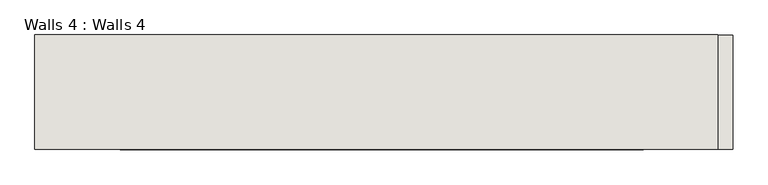
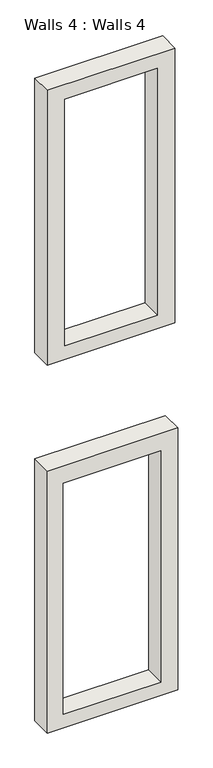
"""IFC4 building model written with IfcOpenShell, lengths in millimetres: wall geometry, Walls 4 : Walls 4."""

from ifc_helpers import new_model, si_unit, frame, origin, place, context, project, spatial, polyline, outline, extrude, source, transform, mapped, element, save


def walls_4_walls_4_8c60a96c(model_context):
    return source(origin(), model_context, "Body", "SweptSolid", [
        extrude(outline(polyline([(6895.2710528, 778.9550968), (6895.2710528, -440.2449032), (4304.4710528, -440.2449032), (4304.4710528, 778.9550968), (6895.2710528, 778.9550968)]), holes=[polyline([(6722.2388367, 622.4491298), (4436.2388367, 622.4491298), (4436.2388367, -291.9508702), (6722.2388367, -291.9508702), (6722.2388367, 622.4491298)])]), frame((0.0, 1354.1985092, 0.0), z_axis=(0.0, 1.0, 0.0), x_axis=(0.0, 0.0, 1.0)), (0.0, 0.0, 1.0), 199.462439),
        extrude(outline(polyline([(10661.4861565, 753.0113734), (10661.4861565, -440.7886266), (7943.6861565, -440.7886266), (7943.6861565, 753.0113734), (10661.4861565, 753.0113734)]), holes=[polyline([(10516.412956, 590.5979517), (8078.012956, 590.5979517), (8078.012956, -276.1770483), (10516.412956, -276.1770483), (10516.412956, 590.5979517)])]), frame((0.0, 1354.1985092, 0.0), z_axis=(0.0, 1.0, 0.0), x_axis=(0.0, 0.0, 1.0)), (0.0, 0.0, 1.0), 199.462439),
    ])


if __name__ == "__main__":
    model = new_model("IFC4")
    model_context = context("Model", 3, world=origin())
    ifc_project = project(units=[si_unit("LENGTHUNIT", "METRE", prefix="MILLI")], contexts=[model_context])
    site = spatial("IfcSite", under=ifc_project)
    building = spatial("IfcBuilding", under=site)
    placement = place(None, origin())
    walls_4_walls_4_shape = walls_4_walls_4_8c60a96c(model_context)
    element("IfcWall", 1, ObjectType="Walls 4 : Walls 4", at=placement, inside=building, context=model_context, shape_type="MappedRepresentation", body=[
        mapped(walls_4_walls_4_shape, transform((0.0, 0.0, 0.0), x_axis=(1.0, 0.0, 0.0), y_axis=(0.0, 1.0, 0.0), z_axis=(0.0, 0.0, 1.0))),
    ])
    save(model, "model.ifc")

# Revit data of these elements
# Element 1 (IfcWall, "Walls 4 : Walls 4")
#   Materials on its faces: "Default Wall"
# Materials
#   "Default Wall": colour RGB 128 128 128, transparency 0
